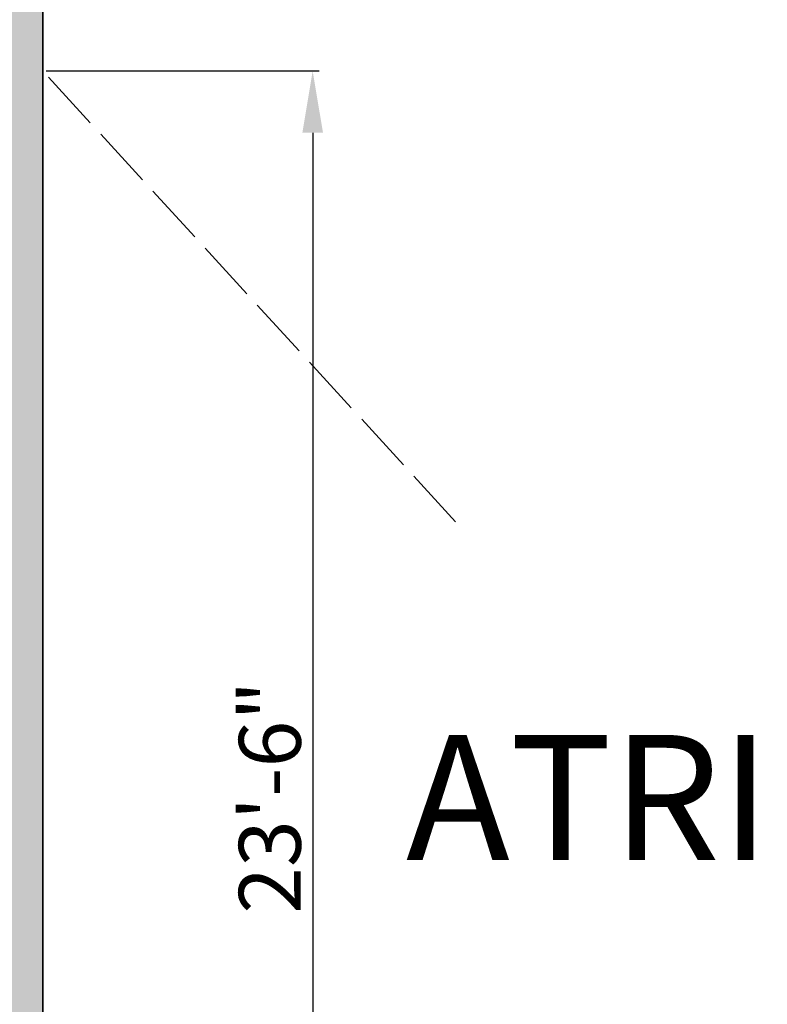
# Model space of a CAD drawing. Units: inches. Extents: x 2083 to 3317, y 1141 to 2115.
# Tile 115 of 256: x 2600 to 2746, y 1522 to 1713. Entities that reach past the tile are written whole.
import ezdxf

# ---------------------------------------------------------------- set-up
doc = ezdxf.new("R2010")
doc.units = ezdxf.units.IN
doc.linetypes.add('ACAD_ISO02W100', pattern=[15, 12, -3])
for name, color, linetype, lineweight in [('A-ANNO-DIMS', 2, 'Continuous', 18), ('A-AREA-IDEN', 7, 'Continuous', 25), ('A-FLOR-OPEN', 8, 'ACAD_ISO02W100', 13), ('A-WALL', 7, 'Continuous', 35)]:
    doc.layers.add(name, color=color, linetype=linetype, lineweight=lineweight)
doc.layers.add('A-WALL-PATT', color=251, linetype='Continuous', lineweight=13, true_color=0x636466)
doc.styles.get("Standard").update_dxf_attribs({"font": 'arial.ttf'})
doc.dimstyles.new('ISO-25', dxfattribs={"dimtxt": 12, "dimasz": 12, "dimexe": 1.25, "dimexo": 0.625, "dimtad": 1, "dimlunit": 3, "dimtxsty": 'Standard', "dimcen": 2.5, "dimadec": 0, "dimazin": 0, "dimtfac": 1, "dimtmove": 0, "dimatfit": 3, "dimfxl": 1, "dimarcsym": 0})

# ---------------------------------------------------------------- blocks, each defined once
blk = doc.blocks.new('*D44')
at = {"layer": 'A-ANNO-DIMS', "color": 0, "lineweight": -2, "transparency": 16777216}
for p, q in [((2605.58, 1702.76), (2658.56, 1702.76)), ((2657.31, 1690.76), (2657.31, 1432.76)), ((2605.58, 1420.76), (2658.56, 1420.76))]:
    blk.add_line(p, q, dxfattribs=at)
at = {"layer": 'A-ANNO-DIMS', "color": 0, "transparency": 16777216}
for points in [[(2655.31, 1690.76), (2659.31, 1690.76), (2657.31, 1702.76)], [(2655.31, 1432.76), (2659.31, 1432.76), (2657.31, 1420.76)]]:
    blk.add_solid(points, dxfattribs=at)
at = {"layer": 'Defpoints', "color": 0, "transparency": 16777216}
for p in [(2604.96, 1702.76), (2604.96, 1420.76), (2657.31, 1420.76)]:
    blk.add_point(p, dxfattribs=at)
at = {"layer": 'A-ANNO-DIMS', "color": 0, "transparency": 16777216, "insert": (2650.55, 1561.76), "char_height": 12, "attachment_point": 5, "rotation": 90}
blk.add_mtext('23\'-6"', dxfattribs=at)

msp = doc.modelspace()

# ---------------------------------------------------------------- hatches: boundary and pattern name
at = {"layer": 'A-WALL-PATT'}
h = msp.add_hatch(color=256, dxfattribs=at)
h.dxf.hatch_style = 1
h.paths.add_polyline_path([(3126.96, 2020.761), (2748.96, 2020.761), (2604.96, 2020.761), (2226.96, 2020.761), (2226.96, 1702.761), (2466.96, 1702.761), (2466.96, 1582.761), (2418.96, 1582.761), (2418.96, 1477.761), (2226.96, 1477.761), (2226.96, 1263.261), (2544.96, 1263.261), (2544.96, 1411.761), (2604.96, 1411.761), (2685.96, 1411.761), (2685.96, 1420.761), (2604.96, 1420.761), (2604.96, 1573.761), (2604.96, 1702.761), (2604.96, 2011.761), (2748.96, 2011.761), (2748.96, 1702.761), (2862.96, 1702.761), (2862.96, 1621.761), (2871.96, 1621.761), (2871.96, 1702.761), (2883.96, 1702.761), (2883.96, 1706.939, -0.0264593), (2883.96, 1711.761), (2757.96, 1711.761), (2757.96, 1807.761), (2787.96, 1807.761), (2787.96, 1812.261), (2757.96, 1812.261), (2757.96, 2011.761), (2877.96, 2011.761), (2877.96, 1812.261), (2847.96, 1812.261), (2847.96, 1807.761), (2889.836, 1807.761), (2889.836, 1812.261), (2882.46, 1812.261), (2882.46, 2011.761), (3117.96, 2011.761), (3117.96, 1812.261), (2937.836, 1812.261), (2937.836, 1807.761), (2995.71, 1807.761), (2995.71, 1796.118), (3000.21, 1796.118), (3000.21, 1807.761), (3117.96, 1807.761), (3117.96, 1711.761), (3000.21, 1711.761), (3000.21, 1760.118), (2998.573, 1760.118, -0.020711), (2995.71, 1760.118), (2995.71, 1711.761), (2931.96, 1711.761), (2931.96, 1702.761), (3126.96, 1702.761)])
h.paths.add_polyline_path([(2471.46, 2011.761), (2471.46, 1810.011), (2462.717, 1810.011), (2462.717, 1805.511), (2505.96, 1805.511), (2505.96, 1810.011), (2475.96, 1810.011), (2475.96, 2011.761), (2595.96, 2011.761), (2595.96, 1810.011), (2565.96, 1810.011), (2565.96, 1805.511), (2595.96, 1805.511), (2595.96, 1711.761), (2235.96, 1711.761), (2235.96, 1805.511), (2353.71, 1805.511), (2353.71, 1796.054), (2358.21, 1796.054), (2358.21, 1805.511), (2414.717, 1805.511), (2414.717, 1810.011), (2235.96, 1810.011), (2235.96, 2011.761)], flags=16)
h.paths.add_polyline_path([(2270.205, 1994.61), (2270.205, 1970.61), (2246.205, 1970.61), (2246.205, 1994.61)], flags=0)
edge = h.paths.add_edge_path(flags=0)
edge.add_ellipse((2332.027, 1899.798), major_axis=(-3.043, 3.043), ratio=0.1682525, start_angle=-161.33217, end_angle=-156.30711, ccw=False)
edge.add_ellipse((2333.082, 1898.744), major_axis=(-1.055, 1.055), ratio=0.4535321, start_angle=-123.37102, end_angle=-94.15911)
edge = h.paths.add_edge_path(flags=0)
edge.add_ellipse((2332.027, 1968.876), major_axis=(3.043, 3.043), ratio=0.1682525, start_angle=18.66783, end_angle=23.69289)
edge.add_spline(control_points=[(2332.926, 1970.691), (2332.227, 1970.336), (2330.894, 1969.659), (2328.413, 1970.932), (2327.204, 1967.749), (2324.71, 1969.956), (2322.533, 1967.012), (2320.013, 1971.296), (2317.68, 1968.158), (2316.041, 1967.102), (2315.427, 1966.81)], knot_values=[0, 0, 0, 0, 2.2670587, 4.3245589, 6.6855835, 8.8786411, 11.121502, 14.300359, 17.7552837, 19.732645, 19.732645, 19.732645, 19.732645], degree=3, periodic=0)
edge.add_ellipse((2332.027, 1968.876), major_axis=(3.043, 3.043), ratio=0.1682525, start_angle=18.66783, end_angle=23.69289, ccw=False)
edge.add_ellipse((2333.082, 1969.931), major_axis=(1.055, 1.055), ratio=0.4535321, start_angle=56.62898, end_angle=85.84089, ccw=False)
edge = h.paths.add_edge_path(flags=0)
edge.add_spline(control_points=[(2296.428, 1967.988), (2293.628, 1965.336), (2287.704, 1959.727), (2299.744, 1949.996), (2294.533, 1935.669), (2290.573, 1920.604), (2293.394, 1909.974), (2296.185, 1904.967)], knot_values=[0.0991853, 0.0991853, 0.0991853, 0.0991853, 0.3453009, 0.6198217, 0.9826526, 1.3860932, 1.8105546, 1.8105546, 1.8105546, 1.8105546], degree=3, periodic=0)
edge.add_spline(control_points=[(2296.185, 1904.967), (2297.384, 1902.619), (2298.001, 1901.949), (2298.553, 1901.468)], knot_values=[0.0062457, 0.0062457, 0.0062457, 0.0062457, 0.0554759, 0.0554759, 0.0554759, 0.0554759], degree=3, periodic=0)
edge.add_spline(control_points=[(2298.553, 1901.468), (2297.259, 1900.923), (2295.225, 1900.232), (2293.06, 1900.614), (2292.101, 1900.788), (2292.09, 1900.791)], knot_values=[0.3128349, 0.3128349, 0.3128349, 0.3128349, 0.4017797, 0.4749867, 0.4759027, 0.4759027, 0.4759027, 0.4759027], degree=3, periodic=0)
edge.add_arc((2292.794, 1904.664), 3.937, 215.4209, 259.69818, ccw=False)
edge.add_spline(control_points=[(2289.585, 1902.382), (2289.477, 1902.535), (2289.368, 1902.688), (2289.261, 1902.841)], knot_values=[0.1028719, 0.1028719, 0.1028719, 0.1028719, 0.1168958, 0.1168958, 0.1168958, 0.1168958], degree=3, periodic=0)
edge.add_spline(control_points=[(2289.261, 1902.841), (2288.687, 1902.55), (2287.64, 1902.02), (2285.881, 1901.874), (2283.853, 1901.504), (2281.72, 1899.711), (2278.467, 1899.493), (2276.157, 1901.883), (2272.259, 1899.804), (2267.778, 1901.843), (2262.244, 1900.184), (2257.415, 1901.782), (2254.318, 1900.726), (2253.178, 1900.337)], knot_values=[0, 0, 0, 0, 1.9079767, 3.4771759, 5.261074, 7.9728515, 11.6802485, 13.7179214, 16.9395917, 22.789562, 27.5025027, 33.5952153, 37.1456181, 37.1456181, 37.1456181, 37.1456181], degree=3, periodic=0)
edge.add_line((2253.178, 1900.337), (2250.244, 1902.841))
edge.add_line((2250.244, 1902.841), (2250.244, 1965.833))
edge.add_line((2250.244, 1965.833), (2253.178, 1968.337))
edge.add_spline(control_points=[(2253.178, 1968.337), (2254.318, 1967.948), (2257.415, 1966.892), (2262.244, 1968.49), (2267.778, 1966.831), (2271.527, 1968.537), (2273.876, 1967.828), (2274.207, 1967.728)], knot_values=[0, 0, 0, 0, 0.0901802, 0.2449351, 0.3646438, 0.5132331, 0.5378548, 0.5378548, 0.5378548, 0.5378548], degree=3, periodic=0)
edge.add_arc((2274.353, 1963.793), 3.937, 72.05113, 92.12795, ccw=False)
edge.add_arc((2281.297, 1985.23), 18.596, 252.05113, 288.56572)
edge.add_arc((2292.317, 1956.029), 12.646, 71.02679, 113.77822, ccw=False)
edge = h.paths.add_edge_path(flags=0)
edge.add_spline(control_points=[(2274.899, 1951.856), (2275.066, 1951.617), (2275.233, 1951.377), (2275.398, 1951.136)], knot_values=[1.4099157, 1.4099157, 1.4099157, 1.4099157, 1.4315903, 1.4315903, 1.4315903, 1.4315903], degree=3, periodic=0)
edge.add_spline(control_points=[(2275.398, 1951.136), (2275.792, 1950.562), (2276.179, 1949.984), (2276.546, 1949.397)], knot_values=[1.3582378, 1.3582378, 1.3582378, 1.3582378, 1.4099157, 1.4099157, 1.4099157, 1.4099157], degree=3, periodic=0)
edge.add_line((2276.546, 1949.397), (2277.437, 1947.862))
edge.add_spline(control_points=[(2277.437, 1947.862), (2276.304, 1945.673), (2274.64, 1942.427), (2274.632, 1938.094), (2272.799, 1930.852), (2274.356, 1943.897), (2275.948, 1947.923), (2276.546, 1949.397)], knot_values=[0.0056315, 0.0056315, 0.0056315, 0.0056315, 0.1860139, 0.2660015, 0.3570872, 0.5963902, 0.7397317, 0.7397317, 0.7397317, 0.7397317], degree=3, periodic=0)
edge.add_spline(control_points=[(2276.546, 1949.397), (2276.179, 1949.984), (2275.792, 1950.562), (2275.398, 1951.136)], knot_values=[1.3582378, 1.3582378, 1.3582378, 1.3582378, 1.4099157, 1.4099157, 1.4099157, 1.4099157], degree=3, periodic=0)
edge.add_spline(control_points=[(2275.398, 1951.136), (2274.943, 1950.08), (2274.208, 1948.025), (2273.935, 1944.851), (2272.469, 1937.627), (2273.466, 1945.696), (2274.701, 1951.059), (2274.899, 1951.856)], knot_values=[0.1043639, 0.1043639, 0.1043639, 0.1043639, 0.1896363, 0.2696239, 0.3607096, 0.6000126, 0.6446217, 0.6446217, 0.6446217, 0.6446217], degree=3, periodic=0)
h.paths.add_polyline_path([(2269.168, 1963.128, -0.3575267), (2268.171, 1960.976, -0.0925607), (2268.171, 1939.436, -0.3575267), (2269.168, 1937.285, -0.3575267), (2267.016, 1938.282, -0.1647847), (2254.686, 1938.282, -0.3575267), (2252.534, 1937.285, -0.3575267), (2253.531, 1939.436, -0.0925607), (2253.531, 1960.976, -0.3575267), (2252.534, 1963.128, -0.3575267), (2254.686, 1962.131, -0.1647847), (2267.016, 1962.131, -0.3575267)], flags=0)
h.paths.add_polyline_path([(2248.874, 1967.802), (2248.874, 1957.028), (2249.458, 1957.028), (2249.458, 1911.647), (2248.874, 1911.647), (2248.874, 1900.873), (2246.512, 1900.873, 0.1973271), (2244.15, 1902.457), (2244.15, 1966.218, 0.1973271), (2246.512, 1967.802)], flags=0)
h.paths.add_polyline_path([(2269.168, 1931.389, -0.3575267), (2268.171, 1929.238, -0.0925607), (2268.171, 1907.698, -0.3575267), (2269.168, 1905.547, -0.3575267), (2267.016, 1906.544, -0.1647847), (2254.686, 1906.544, -0.3575267), (2252.534, 1905.547, -0.3575267), (2253.531, 1907.698, -0.0925607), (2253.531, 1929.238, -0.3575267), (2252.534, 1931.389, -0.3575267), (2254.686, 1930.392, -0.1647847), (2267.016, 1930.392, -0.3575267)], flags=0)
edge = h.paths.add_edge_path(flags=0)
edge.add_spline(control_points=[(2276.197, 1906.724), (2276.168, 1909.029), (2276.114, 1913.372), (2270.598, 1924.925), (2273.905, 1919.013), (2275.922, 1916.262), (2275.475, 1912.402), (2277.258, 1910.381), (2276.696, 1908.225), (2276.646, 1906.813), (2276.618, 1906.008)], knot_values=[0, 0, 0, 0, 8.6102597, 16.2212739, 18.8430575, 23.8048978, 27.4408283, 29.3561016, 31.2034776, 33.6506866, 33.6506866, 33.6506866, 33.6506866], degree=3, periodic=0)
edge.add_spline(control_points=[(2276.618, 1906.008), (2276.623, 1905.624), (2276.498, 1904.629), (2275.442, 1903.855), (2274.937, 1903.08), (2274.859, 1902.841)], knot_values=[0.1564884, 0.1564884, 0.1564884, 0.1564884, 0.1843975, 0.2313765, 0.2505985, 0.2505985, 0.2505985, 0.2505985], degree=3, periodic=0)
edge.add_line((2274.859, 1902.841), (2276.506, 1902.841))
edge.add_spline(control_points=[(2276.506, 1902.841), (2276.788, 1903.085), (2277.665, 1904.125), (2278.25, 1904.341), (2277.654, 1908.527), (2278.156, 1906.228), (2278.1, 1905.286), (2278.847, 1904.069), (2277.857, 1903.415), (2277.874, 1902.991), (2277.904, 1902.841)], knot_values=[0.0595743, 0.0595743, 0.0595743, 0.0595743, 0.0807529, 0.1037415, 0.1697201, 0.1760361, 0.2071372, 0.2404744, 0.2623409, 0.2736605, 0.2736605, 0.2736605, 0.2736605], degree=3, periodic=0)
edge.add_line((2277.904, 1902.841), (2280.03, 1902.841))
edge.add_spline(control_points=[(2280.03, 1902.841), (2279.888, 1903.088), (2279.499, 1903.982), (2280.152, 1905.939), (2278.104, 1909.658), (2279.762, 1907.185), (2280.328, 1904.875), (2280.485, 1903.49), (2281.463, 1903.249), (2281.758, 1902.936), (2281.834, 1902.841)], knot_values=[0.013856, 0.013856, 0.013856, 0.013856, 0.0348738, 0.0888667, 0.1078792, 0.1267378, 0.158714, 0.1937575, 0.2174868, 0.2267221, 0.2267221, 0.2267221, 0.2267221], degree=3, periodic=0)
edge.add_spline(control_points=[(2281.834, 1902.841), (2281.788, 1902.827), (2281.647, 1902.783), (2281.396, 1902.859), (2281.088, 1902.985), (2280.721, 1903.061), (2280.333, 1903.026), (2280.125, 1902.899), (2280.03, 1902.841)], knot_values=[0, 0, 0, 0, 0.1441304, 0.435517, 0.7492759, 1.1530457, 1.5483707, 1.878348, 1.878348, 1.878348, 1.878348], degree=3, periodic=0)
edge.add_line((2280.03, 1902.841), (2277.904, 1902.841))
edge.add_spline(control_points=[(2277.904, 1902.841), (2277.893, 1902.796), (2277.865, 1902.68), (2277.607, 1902.687), (2277.274, 1902.801), (2276.838, 1902.62), (2276.584, 1902.789), (2276.506, 1902.841)], knot_values=[0, 0, 0, 0, 0.1271885, 0.3261988, 0.6280094, 1.2435704, 1.5153306, 1.5153306, 1.5153306, 1.5153306], degree=3, periodic=0)
edge.add_line((2276.506, 1902.841), (2274.859, 1902.841))
edge.add_spline(control_points=[(2274.859, 1902.841), (2274.814, 1902.899), (2274.725, 1903.013), (2274.493, 1903.119), (2274.244, 1902.961), (2273.937, 1903.185), (2273.614, 1902.983), (2273.408, 1902.883), (2273.322, 1902.841)], knot_values=[0, 0, 0, 0, 0.2184302, 0.4369566, 0.6879766, 0.9903786, 1.3983955, 1.6918498, 1.6918498, 1.6918498, 1.6918498], degree=3, periodic=0)
edge.add_spline(control_points=[(2273.322, 1902.841), (2273.617, 1903.446), (2274.274, 1904.538), (2276.027, 1904.574), (2276.207, 1906.584), (2276.197, 1906.724)], knot_values=[0.0122268, 0.0122268, 0.0122268, 0.0122268, 0.0594721, 0.1062177, 0.134458, 0.134458, 0.134458, 0.134458], degree=3, periodic=0)
h.paths.add_polyline_path([(2270.776, 1897.79), (2270.776, 1873.79), (2246.776, 1873.79), (2246.776, 1897.79)], flags=0)
h.paths.add_polyline_path([(2353.71, 1760.005), (2353.71, 1760.054), (2358.21, 1760.054, -0.033729)], flags=0)
h.paths.add_polyline_path([(2321.819, 1737.529), (2341.995, 1737.529, -0.4142136), (2343.203, 1736.321), (2343.203, 1721.021, -0.4142136), (2341.995, 1719.813), (2321.819, 1719.813, -0.4142136), (2320.611, 1721.021), (2320.611, 1736.321, -0.4142136)], flags=0)
h.paths.add_polyline_path([(2324.235, 1736.321), (2339.579, 1736.321, -0.4142136), (2341.995, 1733.905), (2341.995, 1725.45, -0.4142136), (2339.579, 1723.034), (2333.681, 1723.034), (2333.845, 1722.045, -0.8706461), (2335.425, 1721.826, -0.767327), (2333.923, 1721.423), (2331.291, 1721.423, -0.767327), (2329.788, 1721.826, -0.8706461), (2331.368, 1722.045), (2331.533, 1723.034), (2324.235, 1723.034, -0.4142136), (2321.819, 1725.45), (2321.819, 1733.905, -0.4142136)], flags=0)
h.paths.add_polyline_path([(2570.484, 1928.615), (2589.684, 1928.615), (2590.169, 1928.615), (2590.169, 1904.993), (2570.484, 1904.993)], flags=0)
h.paths.add_polyline_path([(2574.447, 1927.264, -1), (2572.829, 1927.264, -1)], flags=0)
h.paths.add_polyline_path([(2573.09, 1926.941), (2573.925, 1927.776), (2574.148, 1927.553), (2573.313, 1926.718)], flags=0)
h.paths.add_polyline_path([(2578.779, 1919.73, -1), (2571.592, 1919.73, -1)], flags=0)
h.paths.add_polyline_path([(2578.385, 1919.73, -1), (2571.985, 1919.73, -1)], flags=0)
h.paths.add_polyline_path([(2331.596, 1729.476, -1), (2333.618, 1729.476, -1)], flags=0)
h.paths.add_polyline_path([(2578.034, 1927.264, -1), (2576.416, 1927.264, -1)], flags=0)
h.paths.add_polyline_path([(2576.689, 1927.531), (2576.912, 1927.754), (2577.747, 1926.919), (2577.524, 1926.696)], flags=0)
h.paths.add_polyline_path([(2578.139, 1909.86, -1), (2572.232, 1909.86, -1)], flags=0)
h.paths.add_polyline_path([(2577.745, 1909.86, -1), (2572.625, 1909.86, -1)], flags=0)
h.paths.add_polyline_path([(2583.798, 1927.264, -1), (2582.179, 1927.264, -1)], flags=0)
h.paths.add_polyline_path([(2582.719, 1927.754), (2583.554, 1926.919), (2583.331, 1926.696), (2582.496, 1927.531)], flags=0)
h.paths.add_polyline_path([(2582.496, 1927.531), (2582.719, 1927.754), (2583.554, 1926.919), (2583.331, 1926.696)], flags=0)
h.paths.add_polyline_path([(2587.739, 1920.53, -1), (2581.832, 1920.53, -1)], flags=0)
h.paths.add_polyline_path([(2587.345, 1920.53, -1), (2582.225, 1920.53, -1)], flags=0)
h.paths.add_polyline_path([(2587.385, 1927.264, -1), (2585.766, 1927.264, -1)], flags=0)
h.paths.add_polyline_path([(2586.082, 1926.98), (2586.917, 1927.815), (2587.14, 1927.593), (2586.305, 1926.758)], flags=0)
h.paths.add_polyline_path([(2588.379, 1910.66, -1), (2581.192, 1910.66, -1)], flags=0)
h.paths.add_polyline_path([(2587.985, 1910.66, -1), (2581.585, 1910.66, -1)], flags=0)
h.paths.add_polyline_path([(2417.168, 1729.478), (2437.344, 1729.478, -0.4142136), (2438.552, 1728.27), (2438.552, 1712.969, -0.4142136), (2437.344, 1711.761), (2417.168, 1711.761, -0.4142136), (2415.96, 1712.969), (2415.96, 1728.27, -0.4142136)], flags=0)
h.paths.add_polyline_path([(2419.584, 1728.27), (2434.928, 1728.27, -0.4142136), (2437.344, 1725.854), (2437.344, 1717.398, -0.4142136), (2434.928, 1714.983), (2429.029, 1714.983), (2429.194, 1713.994, -0.8706461), (2430.774, 1713.775, -0.767327), (2429.271, 1713.372), (2426.64, 1713.372, -0.767327), (2425.137, 1713.775, -0.8706461), (2426.717, 1713.994), (2426.882, 1714.983), (2419.584, 1714.983, -0.4142136), (2417.168, 1717.398), (2417.168, 1725.854, -0.4142136)], flags=0)
h.paths.add_polyline_path([(2419.584, 1728.27), (2434.928, 1728.27, -0.4142136), (2437.344, 1725.854), (2437.344, 1717.398, -0.4142136), (2434.928, 1714.983), (2429.029, 1714.983), (2428.358, 1719.009), (2427.553, 1719.009), (2426.882, 1714.983), (2419.584, 1714.983, -0.4142136), (2417.168, 1717.398), (2417.168, 1725.854, -0.4142136)], flags=0)
h.paths.add_polyline_path([(2426.944, 1721.425, -1), (2428.967, 1721.425, -1)], flags=0)
h.paths.add_polyline_path([(2475.96, 1702.761), (2595.96, 1702.761), (2595.96, 1582.761), (2475.96, 1582.761)], flags=16)
h.paths.add_polyline_path([(2427.96, 1573.761), (2595.96, 1573.761), (2595.96, 1468.761), (2595.96, 1420.761), (2384.46, 1420.761), (2384.46, 1468.761), (2427.96, 1468.761)], flags=16)
h.paths.add_polyline_path([(2379.96, 1468.761), (2379.96, 1420.761), (2235.96, 1420.761), (2235.96, 1468.761)], flags=16)
h.paths.add_polyline_path([(2317.816, 1466.696), (2337.992, 1466.696, -0.4142136), (2339.2, 1465.488), (2339.2, 1450.187, -0.4142136), (2337.992, 1448.979), (2317.816, 1448.979, -0.4142136), (2316.608, 1450.187), (2316.608, 1465.488, -0.4142136)], flags=0)
h.paths.add_polyline_path([(2320.232, 1465.488), (2335.576, 1465.488, -0.4142136), (2337.992, 1463.072), (2337.992, 1454.616, -0.4142136), (2335.576, 1452.2), (2329.677, 1452.2), (2329.842, 1451.212, -0.8706461), (2331.422, 1450.992, -0.767327), (2329.92, 1450.59), (2327.288, 1450.59, -0.767327), (2325.785, 1450.992, -0.8706461), (2327.365, 1451.212), (2327.53, 1452.2), (2320.232, 1452.2, -0.4142136), (2317.816, 1454.616), (2317.816, 1463.072, -0.4142136)], flags=0)
h.paths.add_polyline_path([(2320.232, 1465.488), (2335.576, 1465.488, -0.4142136), (2337.992, 1463.072), (2337.992, 1454.616, -0.4142136), (2335.576, 1452.2), (2329.677, 1452.2), (2329.006, 1456.227), (2328.201, 1456.227), (2327.53, 1452.2), (2320.232, 1452.2, -0.4142136), (2317.816, 1454.616), (2317.816, 1463.072, -0.4142136)], flags=0)
h.paths.add_polyline_path([(2327.593, 1458.643, -1), (2329.615, 1458.643, -1)], flags=0)
h.paths.add_polyline_path([(2244.412, 1433.34), (2241.921, 1433.34, -0.4142136), (2240.018, 1435.244), (2240.018, 1440.953, -0.4142105), (2241.921, 1442.856), (2244.412, 1442.856, -1.9764724)], flags=0)
h.paths.add_polyline_path([(2245.357, 1434.398, -0.4142136), (2245.357, 1441.799, -2.1440985)], flags=0)
h.paths.add_polyline_path([(2535.96, 1416.261), (2535.96, 1272.261), (2235.96, 1272.261), (2235.96, 1416.261)], flags=16)
h.paths.add_polyline_path([(2260.12, 1384.293), (2260.12, 1362.039), (2237.865, 1362.039), (2237.865, 1384.293)], flags=0)
edge = h.paths.add_edge_path(flags=0)
edge.add_line((2318.252, 1362.093), (2318.146, 1362.001))
edge.add_ellipse((2317.445, 1360.431), major_axis=(2.822, 2.822), ratio=0.1682525, start_angle=18.66783, end_angle=20.94813, ccw=False)
edge.add_ellipse((2318.423, 1361.409), major_axis=(0.978, 0.978), ratio=0.4535321, start_angle=56.62898, end_angle=70.2262, ccw=False)
edge = h.paths.add_edge_path(flags=0)
edge.add_line((2319.107, 1295.571), (2319.015, 1295.677))
edge.add_ellipse((2317.445, 1296.378), major_axis=(-2.822, 2.822), ratio=0.1682525, start_angle=-161.33217, end_angle=-159.05187, ccw=False)
edge.add_ellipse((2318.423, 1295.4), major_axis=(-0.978, 0.978), ratio=0.4535321, start_angle=-123.37102, end_angle=-109.7738)
edge = h.paths.add_edge_path(flags=0)
edge.add_spline(control_points=[(2284.21, 1301.17), (2284.581, 1300.445), (2284.891, 1299.892), (2285.16, 1299.461)], knot_values=[0.0390658, 0.0390658, 0.0390658, 0.0390658, 0.0554759, 0.0554759, 0.0554759, 0.0554759], degree=3, periodic=0)
edge.add_line((2285.16, 1299.461), (2284.21, 1301.17))
edge = h.paths.add_edge_path(flags=0)
edge.add_line((2280.412, 1297.298), (2283.37, 1297.036))
edge.add_line((2283.37, 1297.036), (2286.406, 1297.926))
edge.add_spline(control_points=[(2286.406, 1297.926), (2285.305, 1297.463), (2284.345, 1297.129), (2283.37, 1297.036)], knot_values=[0.3943688, 0.3943688, 0.3943688, 0.3943688, 0.4759027, 0.4759027, 0.4759027, 0.4759027], degree=3, periodic=0)
edge.add_spline(control_points=[(2283.37, 1297.036), (2283.281, 1297.028), (2282.316, 1296.957), (2281.313, 1297.134), (2280.423, 1297.296), (2280.412, 1297.298)], knot_values=[0.3128349, 0.3128349, 0.3128349, 0.3128349, 0.3202458, 0.3934528, 0.3943688, 0.3943688, 0.3943688, 0.3943688], degree=3, periodic=0)
edge = h.paths.add_edge_path(flags=0)
edge.add_line((2284.436, 1359.607), (2280.446, 1355.328))
edge.add_line((2280.446, 1355.328), (2279.58, 1351.018))
edge.add_line((2279.58, 1351.018), (2282.413, 1346.58))
edge.add_spline(control_points=[(2282.413, 1346.58), (2283.153, 1345.589), (2284.253, 1344.029), (2284.801, 1342.387), (2284.935, 1341.806)], knot_values=[1.2400982, 1.2400982, 1.2400982, 1.2400982, 1.3328922, 1.3827123, 1.3827123, 1.3827123, 1.3827123], degree=3, periodic=0)
edge.add_spline(control_points=[(2284.935, 1341.806), (2285.319, 1340.141), (2285.233, 1338.409), (2284.91, 1336.654)], knot_values=[1.0974841, 1.0974841, 1.0974841, 1.0974841, 1.2400982, 1.2400982, 1.2400982, 1.2400982], degree=3, periodic=0)
edge.add_spline(control_points=[(2284.91, 1336.654), (2284.587, 1334.899), (2284.027, 1333.12), (2283.463, 1331.361)], knot_values=[0.9548699, 0.9548699, 0.9548699, 0.9548699, 1.0974841, 1.0974841, 1.0974841, 1.0974841], degree=3, periodic=0)
edge.add_line((2283.463, 1331.361), (2281.89, 1326.153))
edge.add_line((2281.89, 1326.153), (2280.756, 1321.056))
edge.add_line((2280.756, 1321.056), (2280.299, 1316.002))
edge.add_line((2280.299, 1316.002), (2280.716, 1310.95))
edge.add_line((2280.716, 1310.95), (2282.028, 1305.972))
edge.add_line((2282.028, 1305.972), (2284.21, 1301.17))
edge.add_spline(control_points=[(2284.21, 1301.17), (2283.341, 1302.73), (2282.612, 1304.336), (2282.028, 1305.972)], knot_values=[0.0991853, 0.0991853, 0.0991853, 0.0991853, 0.2417994, 0.2417994, 0.2417994, 0.2417994], degree=3, periodic=0)
edge.add_spline(control_points=[(2282.028, 1305.972), (2281.444, 1307.608), (2281.005, 1309.273), (2280.716, 1310.95)], knot_values=[0.2417994, 0.2417994, 0.2417994, 0.2417994, 0.3844135, 0.3844135, 0.3844135, 0.3844135], degree=3, periodic=0)
edge.add_spline(control_points=[(2280.716, 1310.95), (2280.433, 1312.588), (2280.289, 1314.277), (2280.299, 1315.962), (2280.299, 1316.002)], knot_values=[0.3844135, 0.3844135, 0.3844135, 0.3844135, 0.5236467, 0.5270276, 0.5270276, 0.5270276, 0.5270276], degree=3, periodic=0)
edge.add_spline(control_points=[(2280.299, 1316.002), (2280.312, 1317.687), (2280.478, 1319.368), (2280.756, 1321.056)], knot_values=[0.5270276, 0.5270276, 0.5270276, 0.5270276, 0.6696417, 0.6696417, 0.6696417, 0.6696417], degree=3, periodic=0)
edge.add_spline(control_points=[(2280.756, 1321.056), (2281.035, 1322.744), (2281.426, 1324.44), (2281.89, 1326.153)], knot_values=[0.6696417, 0.6696417, 0.6696417, 0.6696417, 0.8122558, 0.8122558, 0.8122558, 0.8122558], degree=3, periodic=0)
edge.add_spline(control_points=[(2281.89, 1326.153), (2282.264, 1327.533), (2282.788, 1329.262), (2283.353, 1331.018), (2283.463, 1331.361)], knot_values=[0.8122558, 0.8122558, 0.8122558, 0.8122558, 0.9270873, 0.9548699, 0.9548699, 0.9548699, 0.9548699], degree=3, periodic=0)
edge.add_line((2283.463, 1331.361), (2284.91, 1336.654))
edge.add_line((2284.91, 1336.654), (2284.935, 1341.806))
edge.add_line((2284.935, 1341.806), (2282.413, 1346.58))
edge.add_spline(control_points=[(2282.413, 1346.58), (2281.275, 1348.104), (2280.078, 1349.57), (2279.58, 1351.018)], knot_values=[1.3827123, 1.3827123, 1.3827123, 1.3827123, 1.5253264, 1.5253264, 1.5253264, 1.5253264], degree=3, periodic=0)
edge.add_spline(control_points=[(2279.58, 1351.018), (2279.443, 1351.415), (2279.136, 1352.857), (2279.735, 1354.29), (2280.446, 1355.328)], knot_values=[1.5253264, 1.5253264, 1.5253264, 1.5253264, 1.564439, 1.6679405, 1.6679405, 1.6679405, 1.6679405], degree=3, periodic=0)
edge.add_spline(control_points=[(2280.446, 1355.328), (2281.426, 1356.758), (2282.931, 1358.183), (2284.436, 1359.607)], knot_values=[1.6679405, 1.6679405, 1.6679405, 1.6679405, 1.8105546, 1.8105546, 1.8105546, 1.8105546], degree=3, periodic=0)
edge.add_arc((2280.623, 1348.518), 11.726, 71.02679, 113.77822)
edge.add_arc((2270.405, 1375.595), 17.244, 252.05113, 288.56572, ccw=False)
edge.add_arc((2263.966, 1355.718), 3.651, 72.05113, 92.12795)
edge.add_arc((2263.966, 1355.718), 3.651, 92.12795, 177.98513)
edge.add_spline(control_points=[(2260.318, 1355.846), (2260.26, 1354.221), (2260.551, 1350.187), (2262.999, 1346.766), (2264.473, 1344.649)], knot_values=[1.4315903, 1.4315903, 1.4315903, 1.4315903, 1.5641438, 1.7706953, 1.7706953, 1.7706953, 1.7706953], degree=3, periodic=0)
edge.add_line((2264.473, 1344.649), (2264.936, 1343.983))
edge.add_spline(control_points=[(2263.801, 1340.248), (2263.843, 1340.514), (2264.067, 1341.756), (2264.513, 1343.002), (2264.935, 1343.981)], knot_values=[0.5365702, 0.5365702, 0.5365702, 0.5365702, 0.5593494, 0.6446217, 0.6446217, 0.6446217, 0.6446217], degree=3, periodic=0)
edge.add_spline(control_points=[(2264.935, 1343.981), (2265.118, 1343.715), (2265.299, 1343.448), (2265.477, 1343.179)], knot_values=[1.3840767, 1.3840767, 1.3840767, 1.3840767, 1.4099157, 1.4099157, 1.4099157, 1.4099157], degree=3, periodic=0)
edge.add_spline(control_points=[(2265.477, 1343.179), (2265.655, 1342.911), (2265.829, 1342.641), (2265.999, 1342.369)], knot_values=[1.3582378, 1.3582378, 1.3582378, 1.3582378, 1.3840767, 1.3840767, 1.3840767, 1.3840767], degree=3, periodic=0)
edge.add_line((2265.999, 1342.369), (2266.826, 1340.946))
edge.add_spline(control_points=[(2266.826, 1340.946), (2268.894, 1337.09), (2271.398, 1325.843), (2270.516, 1310.569), (2275.919, 1301.861), (2277.79, 1299.199)], knot_values=[0.1168958, 0.1168958, 0.1168958, 0.1168958, 0.4729873, 1.0509689, 1.3137934, 1.3137934, 1.3137934, 1.3137934], degree=3, periodic=0)
edge.add_spline(control_points=[(2277.79, 1299.199), (2277.839, 1299.128), (2277.889, 1299.057), (2277.94, 1298.987)], knot_values=[0.1098839, 0.1098839, 0.1098839, 0.1098839, 0.1168958, 0.1168958, 0.1168958, 0.1168958], degree=3, periodic=0)
edge.add_line((2277.94, 1298.987), (2277.789, 1299.199))
edge.add_spline(control_points=[(2277.789, 1299.199), (2277.257, 1298.929), (2276.286, 1298.438), (2275.039, 1298.334), (2274.383, 1298.239), (2274.215, 1298.209)], knot_values=[33.1218702, 33.1218702, 33.1218702, 33.1218702, 35.0290557, 36.5982549, 37.1448269, 37.1448269, 37.1448269, 37.1448269], degree=3, periodic=0)
edge.add_line((2274.215, 1298.209), (2273.073, 1297.893))
edge.add_spline(control_points=[(2273.073, 1297.893), (2272.323, 1297.58), (2271.039, 1296.511), (2269.248, 1296.226), (2268.423, 1296.375)], knot_values=[26.5325843, 26.5325843, 26.5325843, 26.5325843, 29.198919, 31.8391012, 31.8391012, 31.8391012, 31.8391012], degree=3, periodic=0)
edge.add_line((2268.423, 1296.375), (2263.879, 1297.458))
edge.add_spline(control_points=[(2263.879, 1297.458), (2263.556, 1297.359), (2261.86, 1296.839), (2260.239, 1297.282), (2258.933, 1297.516)], knot_values=[15.9195506, 15.9195506, 15.9195506, 15.9195506, 16.9395917, 21.2260675, 21.2260675, 21.2260675, 21.2260675], degree=3, periodic=0)
edge.add_line((2258.933, 1297.516), (2254.055, 1297.329))
edge.add_spline(control_points=[(2254.055, 1297.329), (2253.756, 1297.296), (2252.114, 1297.165), (2250.462, 1297.544), (2249.13, 1297.668)], knot_values=[5.3065169, 5.3065169, 5.3065169, 5.3065169, 6.2764352, 10.6130337, 10.6130337, 10.6130337, 10.6130337], degree=3, periodic=0)
edge.add_line((2249.13, 1297.668), (2244.332, 1296.878))
edge.add_line((2244.332, 1296.878), (2241.611, 1299.199))
edge.add_line((2241.611, 1299.199), (2241.611, 1357.609))
edge.add_line((2241.611, 1357.609), (2244.332, 1359.931))
edge.add_line((2244.332, 1359.931), (2252.729, 1359.543))
edge.add_spline(control_points=[(2252.729, 1359.543), (2252.871, 1359.546), (2253.306, 1359.548), (2253.74, 1359.514), (2254.032, 1359.482)], knot_values=[0.233291, 0.233291, 0.233291, 0.233291, 0.2449351, 0.2689274, 0.2689274, 0.2689274, 0.2689274], degree=3, periodic=0)
edge.add_line((2254.032, 1359.482), (2259.587, 1359.416))
edge.add_spline(control_points=[(2259.587, 1359.416), (2260.677, 1359.629), (2262.073, 1359.897), (2263.524, 1359.459), (2263.83, 1359.366)], knot_values=[0.4225164, 0.4225164, 0.4225164, 0.4225164, 0.5132331, 0.5378548, 0.5378548, 0.5378548, 0.5378548], degree=3, periodic=0)
edge.add_arc((2263.966, 1355.718), 3.651, 72.05113, 92.12795, ccw=False)
edge.add_arc((2270.405, 1375.595), 17.244, 252.05113, 288.56572)
edge.add_arc((2280.623, 1348.518), 11.726, 71.02679, 113.77822, ccw=False)
h.paths.add_polyline_path([(2240.341, 1359.435), (2240.341, 1349.444), (2240.882, 1349.444), (2240.882, 1307.365), (2240.341, 1307.365), (2240.341, 1297.374), (2238.15, 1297.374, 0.1973271), (2235.96, 1298.843), (2235.96, 1357.966, 0.1973271), (2238.15, 1359.435)], flags=0)
h.paths.add_polyline_path([(2259.158, 1355.101, -0.3575267), (2258.233, 1353.106, -0.0925607), (2258.233, 1333.133, -0.3575267), (2259.158, 1331.138, -0.3575267), (2257.163, 1332.062, -0.1647847), (2245.729, 1332.062, -0.3575267), (2243.735, 1331.138, -0.3575267), (2244.659, 1333.133, -0.0925607), (2244.659, 1353.106, -0.3575267), (2243.735, 1355.101, -0.3575267), (2245.729, 1354.176, -0.1647847), (2257.163, 1354.176, -0.3575267)], flags=0)
edge = h.paths.add_edge_path(flags=0)
edge.add_line((2265.999, 1342.369), (2266.826, 1340.946))
edge.add_line((2266.826, 1340.946), (2265.308, 1337.814))
edge.add_line((2265.308, 1337.814), (2264.358, 1334.653))
edge.add_line((2264.358, 1334.653), (2264.262, 1333.8))
edge.add_spline(control_points=[(2264.262, 1333.8), (2264.208, 1333.187), (2264.162, 1332.366), (2264.007, 1331.414), (2263.969, 1331.202)], knot_values=[0.4644442, 0.4644442, 0.4644442, 0.4644442, 0.5166905, 0.5316081, 0.5316081, 0.5316081, 0.5316081], degree=3, periodic=0)
edge.add_spline(control_points=[(2263.969, 1331.202), (2263.775, 1330.119), (2263.424, 1328.791), (2263.257, 1328.531), (2263.234, 1328.515)], knot_values=[0.3726816, 0.3726816, 0.3726816, 0.3726816, 0.4488497, 0.4644442, 0.4644442, 0.4644442, 0.4644442], degree=3, periodic=0)
edge.add_spline(control_points=[(2263.234, 1328.515), (2263.096, 1328.42), (2263.131, 1329.301), (2263.275, 1330.616)], knot_values=[0.2809191, 0.2809191, 0.2809191, 0.2809191, 0.3726816, 0.3726816, 0.3726816, 0.3726816], degree=3, periodic=0)
edge.add_spline(control_points=[(2263.275, 1330.616), (2263.419, 1331.93), (2263.672, 1333.677), (2263.97, 1335.315)], knot_values=[0.1891566, 0.1891566, 0.1891566, 0.1891566, 0.2809191, 0.2809191, 0.2809191, 0.2809191], degree=3, periodic=0)
edge.add_spline(control_points=[(2263.97, 1335.315), (2264.1, 1336.032), (2264.419, 1337.622), (2264.755, 1338.864), (2264.947, 1339.491)], knot_values=[0.097394, 0.097394, 0.097394, 0.097394, 0.1375775, 0.1891566, 0.1891566, 0.1891566, 0.1891566], degree=3, periodic=0)
edge.add_spline(control_points=[(2264.947, 1339.491), (2265.29, 1340.606), (2265.644, 1341.494), (2265.999, 1342.369)], knot_values=[0.0056315, 0.0056315, 0.0056315, 0.0056315, 0.097394, 0.097394, 0.097394, 0.097394], degree=3, periodic=0)
h.paths.add_polyline_path([(2259.158, 1325.671, -0.3575267), (2258.233, 1323.676, -0.0925607), (2258.233, 1303.703, -0.3575267), (2259.158, 1301.708, -0.3575267), (2257.163, 1302.633, -0.1647847), (2245.729, 1302.633, -0.3575267), (2243.735, 1301.708, -0.3575267), (2244.659, 1303.703, -0.0925607), (2244.659, 1323.676, -0.3575267), (2243.735, 1325.671, -0.3575267), (2245.729, 1324.747, -0.1647847), (2257.163, 1324.747, -0.3575267)], flags=0)
edge = h.paths.add_edge_path(flags=0)
edge.add_spline(control_points=[(2261.709, 1317.311), (2261.679, 1317.418), (2261.762, 1317.389), (2262.491, 1316.09), (2262.962, 1315.301)], knot_values=[14.9558607, 14.9558607, 14.9558607, 14.9558607, 16.2212739, 18.6948259, 18.6948259, 18.6948259, 18.6948259], degree=3, periodic=0)
edge.add_spline(control_points=[(2262.962, 1315.301), (2262.99, 1315.254), (2263.702, 1314.067), (2264.349, 1313.127), (2264.73, 1312.164)], knot_values=[18.6948259, 18.6948259, 18.6948259, 18.6948259, 18.8430575, 22.433791, 22.433791, 22.433791, 22.433791], degree=3, periodic=0)
edge.add_spline(control_points=[(2264.73, 1312.164), (2264.876, 1311.796), (2265.177, 1310.77), (2265.143, 1309.559), (2265.248, 1308.824)], knot_values=[22.433791, 22.433791, 22.433791, 22.433791, 23.8048978, 26.1727562, 26.1727562, 26.1727562, 26.1727562], degree=3, periodic=0)
edge.add_line((2265.248, 1308.824), (2265.851, 1307.172))
edge.add_spline(control_points=[(2265.851, 1307.172), (2266.065, 1306.822), (2266.384, 1306.332), (2266.424, 1305.781), (2266.42, 1305.611)], knot_values=[28.0625624, 28.0625624, 28.0625624, 28.0625624, 29.3561016, 29.9117214, 29.9117214, 29.9117214, 29.9117214], degree=3, periodic=0)
edge.add_spline(control_points=[(2266.42, 1305.611), (2266.416, 1305.433), (2266.394, 1305.25), (2266.365, 1305.066)], knot_values=[29.9117214, 29.9117214, 29.9117214, 29.9117214, 30.4978371, 30.4978371, 30.4978371, 30.4978371], degree=3, periodic=0)
edge.add_line((2266.365, 1305.066), (2266.066, 1302.136))
edge.add_spline(control_points=[(2266.066, 1302.136), (2266.071, 1301.78), (2265.998, 1301.2), (2265.663, 1300.759), (2265.509, 1300.586)], knot_values=[0.1564884, 0.1564884, 0.1564884, 0.1564884, 0.1843975, 0.2035434, 0.2035434, 0.2035434, 0.2035434], degree=3, periodic=0)
edge.add_line((2265.509, 1300.586), (2264.435, 1299.199))
edge.add_line((2264.435, 1299.199), (2265.962, 1299.199))
edge.add_line((2265.962, 1299.199), (2267.336, 1301.175))
edge.add_line((2267.336, 1301.175), (2267.312, 1301.986))
edge.add_spline(control_points=[(2267.312, 1301.986), (2267.261, 1302.862), (2267.16, 1303.737), (2267.271, 1303.326)], knot_values=[0.1262286, 0.1262286, 0.1262286, 0.1262286, 0.1666174, 0.1666174, 0.1666174, 0.1666174], degree=3, periodic=0)
edge.add_spline(control_points=[(2267.271, 1303.326), (2267.28, 1303.294), (2267.31, 1303.175), (2267.373, 1302.884), (2267.406, 1302.683), (2267.418, 1302.601)], knot_values=[0.1666174, 0.1666174, 0.1666174, 0.1666174, 0.1697201, 0.1760361, 0.1807647, 0.1807647, 0.1807647, 0.1807647], degree=3, periodic=0)
edge.add_spline(control_points=[(2267.744, 1300.988), (2267.688, 1301.151), (2267.481, 1301.657), (2267.484, 1302.145), (2267.418, 1302.601)], knot_values=[0.1807647, 0.1807647, 0.1807647, 0.1807647, 0.1937665, 0.2201389, 0.2201389, 0.2201389, 0.2201389], degree=3, periodic=0)
edge.add_line((2267.418, 1302.601), (2267.744, 1300.988))
edge.add_spline(control_points=[(2267.744, 1300.988), (2267.832, 1300.732), (2267.932, 1300.31), (2267.555, 1299.975), (2267.429, 1299.829)], knot_values=[0.2201389, 0.2201389, 0.2201389, 0.2201389, 0.2404744, 0.2548903, 0.2548903, 0.2548903, 0.2548903], degree=3, periodic=0)
edge.add_line((2267.429, 1299.829), (2267.258, 1299.199))
edge.add_line((2267.258, 1299.199), (2269.23, 1299.199))
edge.add_spline(control_points=[(2269.23, 1299.199), (2269.099, 1299.429), (2268.843, 1300.016), (2269.012, 1300.916), (2268.947, 1301.661)], knot_values=[0.013856, 0.013856, 0.013856, 0.013856, 0.0348738, 0.0670726, 0.0670726, 0.0670726, 0.0670726], degree=3, periodic=0)
edge.add_line((2268.947, 1301.661), (2268.432, 1303.603))
edge.add_spline(control_points=[(2268.432, 1303.603), (2268.176, 1304.192), (2267.596, 1305.251), (2268.041, 1304.623), (2268.251, 1304.282)], knot_values=[0.0901547, 0.0901547, 0.0901547, 0.0901547, 0.1078792, 0.1202891, 0.1202891, 0.1202891, 0.1202891], degree=3, periodic=0)
edge.add_spline(control_points=[(2268.251, 1304.282), (2268.361, 1304.105), (2269.058, 1302.918), (2269.383, 1301.59), (2269.521, 1300.776), (2269.575, 1300.556)], knot_values=[0.1202891, 0.1202891, 0.1202891, 0.1202891, 0.1267378, 0.158714, 0.1735056, 0.1735056, 0.1735056, 0.1735056], degree=3, periodic=0)
edge.add_line((2269.575, 1300.556), (2270.686, 1299.421))
edge.add_spline(control_points=[(2270.686, 1299.421), (2270.767, 1299.357), (2270.838, 1299.281), (2270.903, 1299.199)], knot_values=[0.2181597, 0.2181597, 0.2181597, 0.2181597, 0.2267221, 0.2267221, 0.2267221, 0.2267221], degree=3, periodic=0)
edge.add_line((2270.937, 1299.193), (2270.903, 1299.199))
edge.add_spline(control_points=[(2270.903, 1299.199), (2270.86, 1299.186), (2270.73, 1299.146), (2270.496, 1299.216), (2270.272, 1299.308), (2270.121, 1299.348), (2270.063, 1299.36)], knot_values=[0.939174, 0.939174, 0.939174, 0.939174, 1.0833044, 1.3746911, 1.6884499, 1.878348, 1.878348, 1.878348, 1.878348], degree=3, periodic=0)
edge.add_line((2270.063, 1299.36), (2269.23, 1299.199))
edge.add_line((2269.23, 1299.199), (2267.258, 1299.199))
edge.add_spline(control_points=[(2267.258, 1299.199), (2267.248, 1299.157), (2267.223, 1299.05), (2266.984, 1299.057), (2266.809, 1299.116), (2266.677, 1299.109), (2266.637, 1299.105)], knot_values=[0.7576653, 0.7576653, 0.7576653, 0.7576653, 0.8848538, 1.0838641, 1.3856747, 1.5153306, 1.5153306, 1.5153306, 1.5153306], degree=3, periodic=0)
edge.add_spline(control_points=[(2266.637, 1299.105), (2266.485, 1299.089), (2266.236, 1299.017), (2266.035, 1299.151), (2265.962, 1299.199)], knot_values=[0, 0, 0, 0, 0.4859051, 0.7576653, 0.7576653, 0.7576653, 0.7576653], degree=3, periodic=0)
edge.add_line((2265.962, 1299.199), (2264.435, 1299.199))
edge.add_line((2264.435, 1299.199), (2263.858, 1299.367))
edge.add_spline(control_points=[(2263.858, 1299.367), (2263.819, 1299.371), (2263.78, 1299.386), (2263.74, 1299.402)], knot_values=[0.8459249, 0.8459249, 0.8459249, 0.8459249, 0.9786272, 0.9786272, 0.9786272, 0.9786272], degree=3, periodic=0)
edge.add_line((2263.722, 1299.396), (2263.01, 1299.199))
edge.add_spline(control_points=[(2263.01, 1299.199), (2263.246, 1299.683), (2263.506, 1300.128), (2263.873, 1300.408)], knot_values=[0.0122268, 0.0122268, 0.0122268, 0.0122268, 0.0529705, 0.0529705, 0.0529705, 0.0529705], degree=3, periodic=0)
edge.add_spline(control_points=[(2263.873, 1300.408), (2263.932, 1300.453), (2264.084, 1300.553), (2264.255, 1300.624), (2264.36, 1300.665)], knot_values=[0.0529705, 0.0529705, 0.0529705, 0.0529705, 0.0594721, 0.0690861, 0.0690861, 0.0690861, 0.0690861], degree=3, periodic=0)
edge.add_line((2264.36, 1300.665), (2265.142, 1301.078))
edge.add_line((2265.142, 1301.078), (2265.676, 1302.8))
edge.add_line((2265.676, 1302.8), (2265.541, 1305.704))
edge.add_line((2265.541, 1305.704), (2264.803, 1309.328))
edge.add_line((2264.803, 1309.328), (2263.041, 1314.092))
edge.add_spline(control_points=[(2263.041, 1314.092), (2262.384, 1315.671), (2261.796, 1316.998), (2261.709, 1317.311)], knot_values=[11.2168955, 11.2168955, 11.2168955, 11.2168955, 14.9558607, 14.9558607, 14.9558607, 14.9558607], degree=3, periodic=0)
h.paths.add_polyline_path([(2871.96, 1416.261), (2895.91, 1416.261), (2895.91, 1420.761), (2871.96, 1420.761), (2871.96, 1501.761), (2862.96, 1501.761), (2862.96, 1420.761), (2805.96, 1420.761), (2805.96, 1411.761), (2862.96, 1411.761), (2862.96, 1263.261), (3126.96, 1263.261), (3126.96, 1411.761), (3126.96, 1486.761), (2943.96, 1486.761), (2943.96, 1477.761), (2967.86, 1477.761), (2967.86, 1420.761), (2943.91, 1420.761), (2943.91, 1416.261), (3117.96, 1416.261), (3117.96, 1420.761), (2972.36, 1420.761), (2972.36, 1477.761), (3117.96, 1477.761), (3117.96, 1420.761), (3117.96, 1272.261), (2871.96, 1272.261)], flags=0)
h.paths.add_polyline_path([(2457.126, 1485.943), (2527.603, 1485.943), (2527.603, 1537.636), (2457.126, 1537.636)], flags=8)
h.paths.add_polyline_path([(2481.005, 1609.982), (2590.766, 1609.982), (2590.766, 1682.003), (2481.005, 1682.003)], flags=8)
h.paths.add_polyline_path([(2483.085, 1729.127), (2553.562, 1729.127), (2553.562, 1780.82), (2483.085, 1780.82)], flags=8)

# ---------------------------------------------------------------- linework, layer by layer
at = {"layer": 'A-FLOR-OPEN'}
msp.add_line((2685.041, 1615.231), (2604.96, 1702.761), dxfattribs=at)
at = {"layer": 'A-WALL'}
for p, q in [((2604.96, 2011.761), (2604.96, 1702.761)), ((2604.96, 1702.761), (2604.96, 1573.761)), ((2604.96, 1573.761), (2604.96, 1420.761))]:
    msp.add_line(p, q, dxfattribs=at)

# ---------------------------------------------------------------- texts
at = {"layer": 'A-AREA-IDEN', "insert": (2675.425, 1573.845), "char_height": 24.2645, "attachment_point": 1}
msp.add_mtext_dynamic_manual_height_columns('ATRIUM', width=440.66147, gutter_width=121.322, heights=[0], dxfattribs=at)

# ---------------------------------------------------------------- dimensions: what is measured, and where the dimension line sits
at = {"layer": 'A-ANNO-DIMS'}
dim = msp.add_linear_dim(base=(2657.31, 1420.761), p1=(2604.96, 1702.761), p2=(2604.96, 1420.761), angle=270, dimstyle='ISO-25', override={"dimdec": 1, "dimlfac": 1, "dimrnd": 0, "dimzin": 1, "dimdsep": 46, "dimlunit": 4, "dimfrac": 2}, dxfattribs=at)
dim.commit()
dim.dimension.update_dxf_attribs({"geometry": '*D44', "text_midpoint": (2650.554, 1561.761)})

doc.saveas('drawing.dxf')
